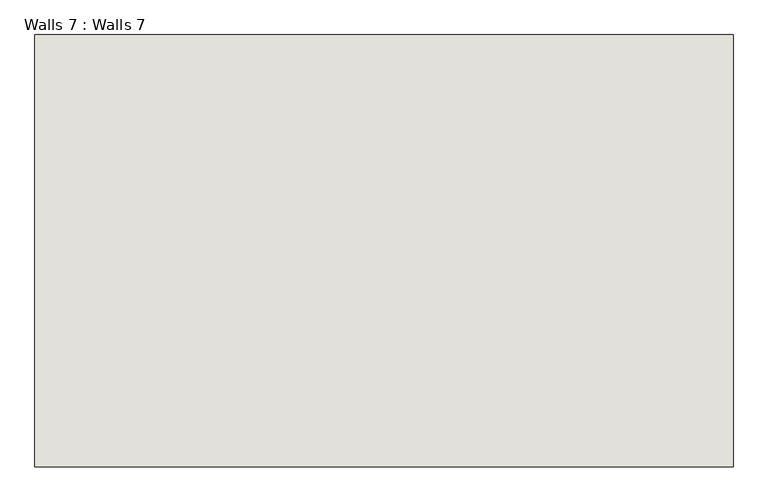
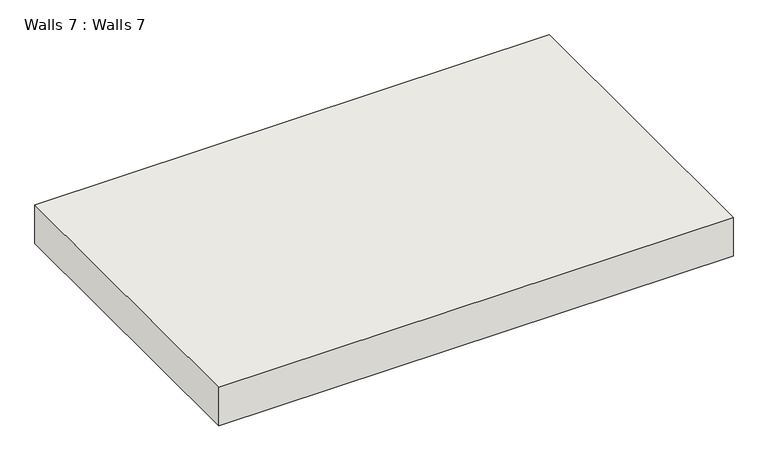
"""IFC4 building model written with IfcOpenShell, lengths in millimetres: wall geometry, Walls 7 : Walls 7."""

from ifc_helpers import new_model, si_unit, frame, origin, place, context, project, spatial, polyline, outline, extrude, source, transform, mapped, element, save


def walls_7_walls_7_1d2fd38e(model_context):
    return source(origin(), model_context, "Body", "SweptSolid", [
        extrude(outline(polyline([(-9784.4289001, -3697.5103614), (-13639.064077, -3697.5103614), (-13639.064077, -1309.7180898), (-9784.4289001, -1309.7180898), (-9784.4289001, -3697.5103614)])), frame((0.0, 0.0, 6096.0), z_axis=(0.0, 0.0, 1.0), x_axis=(1.0, 0.0, 0.0)), (0.0, 0.0, 1.0), 304.8),
    ])


if __name__ == "__main__":
    model = new_model("IFC4")
    model_context = context("Model", 3, world=origin())
    ifc_project = project(units=[si_unit("LENGTHUNIT", "METRE", prefix="MILLI")], contexts=[model_context])
    site = spatial("IfcSite", under=ifc_project)
    building = spatial("IfcBuilding", under=site)
    placement = place(None, origin())
    walls_7_walls_7_shape = walls_7_walls_7_1d2fd38e(model_context)
    element("IfcWall", 1, ObjectType="Walls 7 : Walls 7", at=placement, inside=building, context=model_context, shape_type="MappedRepresentation", body=[
        mapped(walls_7_walls_7_shape, transform((0.0, 0.0, 0.0), x_axis=(1.0, 0.0, 0.0), y_axis=(0.0, 1.0, 0.0), z_axis=(0.0, 0.0, 1.0))),
    ])
    save(model, "model.ifc")

# Revit data of these elements
# Element 1 (IfcWall, "Walls 7 : Walls 7")
#   Materials on its faces: "Default Wall"
# Materials
#   "Default Wall": colour RGB 80 80 80, transparency 0
